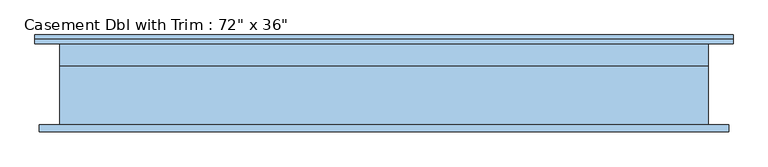
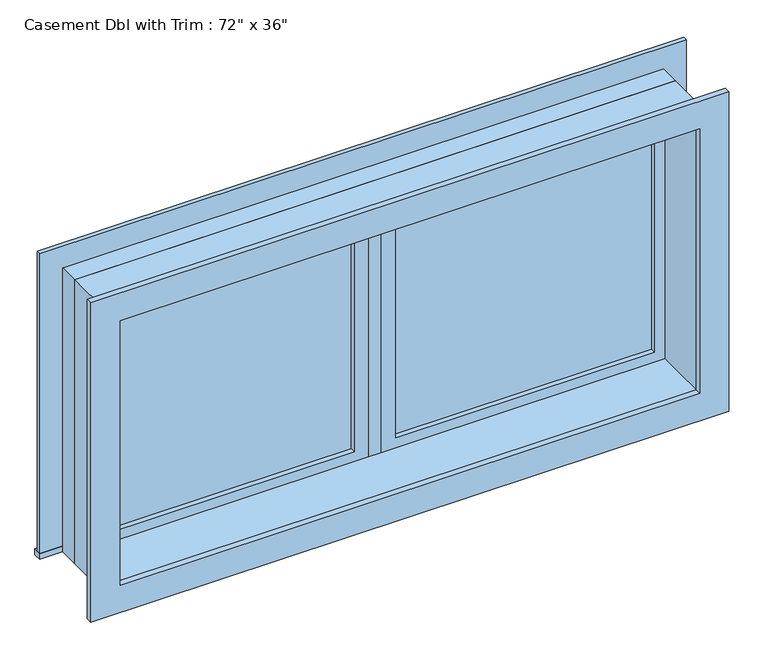
"""IFC4 building model written with IfcOpenShell, lengths in millimetres: window geometry."""

from ifc_helpers import new_model, si_unit, frame, origin, place, context, project, spatial, polyline, outline, extrude, source, transform, mapped, element, save


def window_6788402d(model_context):
    return source(origin(), model_context, "Body", "SweptSolid", [
        extrude(outline(polyline([(63.5, 98.425), (850.9, 98.425), (850.9, 85.725), (63.5, 85.725), (63.5, 98.425)])), frame((0.0, 0.0, 1282.7), z_axis=(0.0, 0.0, 1.0), x_axis=(1.0, 0.0, 0.0)), (0.0, 0.0, 1.0), 787.4),
        extrude(outline(polyline([(2114.55, 19.05), (1238.25, 19.05), (1238.25, 895.35), (2114.55, 895.35), (2114.55, 19.05)]), holes=[polyline([(2070.1, 63.5), (2070.1, 850.9), (1282.7, 850.9), (1282.7, 63.5), (2070.1, 63.5)])]), frame((0.0, 69.85, 0.0), z_axis=(0.0, 1.0, 0.0), x_axis=(0.0, 0.0, 1.0)), (0.0, 0.0, 1.0), 44.45),
        extrude(outline(polyline([(19.05, 69.85), (-19.05, 69.85), (-19.05, 133.35), (19.05, 133.35), (19.05, 69.85)])), frame((0.0, 0.0, 1238.25), z_axis=(0.0, 0.0, 1.0), x_axis=(1.0, 0.0, 0.0)), (0.0, 0.0, 1.0), 876.3),
        extrude(outline(polyline([(-984.25, 158.75), (984.25, 158.75), (984.25, 133.35), (-984.25, 133.35), (-984.25, 158.75)])), frame((0.0, 0.0, 1219.2), z_axis=(0.0, 0.0, 1.0), x_axis=(1.0, 0.0, 0.0)), (0.0, 0.0, 1.0), 19.05),
        extrude(outline(polyline([(2114.55, -895.35), (2114.55, 895.35), (1238.25, 895.35), (1238.25, 984.25), (2203.45, 984.25), (2203.45, -984.25), (1238.25, -984.25), (1238.25, -895.35), (2114.55, -895.35)])), frame((0.0, 133.35, 0.0), z_axis=(0.0, 1.0, 0.0), x_axis=(0.0, 0.0, 1.0)), (0.0, 0.0, 1.0), 12.7),
        extrude(outline(polyline([(2190.75, 971.55), (2190.75, -971.55), (1162.05, -971.55), (1162.05, 971.55), (2190.75, 971.55)]), holes=[polyline([(2101.85, 882.65), (1250.95, 882.65), (1250.95, -882.65), (2101.85, -882.65), (2101.85, 882.65)])]), frame((0.0, -114.3, 0.0), z_axis=(0.0, 1.0, 0.0), x_axis=(0.0, 0.0, 1.0)), (0.0, 0.0, 1.0), 19.05),
        extrude(outline(polyline([(-63.5, 85.725), (-850.9, 85.725), (-850.9, 98.425), (-63.5, 98.425), (-63.5, 85.725)])), frame((0.0, 0.0, 1282.7), z_axis=(0.0, 0.0, 1.0), x_axis=(1.0, 0.0, 0.0)), (0.0, 0.0, 1.0), 787.4),
        extrude(outline(polyline([(2114.55, -895.35), (1238.25, -895.35), (1238.25, -19.05), (2114.55, -19.05), (2114.55, -895.35)]), holes=[polyline([(2070.1, -850.9), (2070.1, -63.5), (1282.7, -63.5), (1282.7, -850.9), (2070.1, -850.9)])]), frame((0.0, 69.85, 0.0), z_axis=(0.0, 1.0, 0.0), x_axis=(0.0, 0.0, 1.0)), (0.0, 0.0, 1.0), 44.45),
        extrude(outline(polyline([(2133.6, -914.4), (1219.2, -914.4), (1219.2, 914.4), (2133.6, 914.4), (2133.6, -914.4)]), holes=[polyline([(2101.85, -882.65), (2101.85, 882.65), (1250.95, 882.65), (1250.95, -882.65), (2101.85, -882.65)])]), frame((0.0, -95.25, 0.0), z_axis=(0.0, 1.0, 0.0), x_axis=(0.0, 0.0, 1.0)), (0.0, 0.0, 1.0), 165.1),
        extrude(outline(polyline([(2133.6, 914.4), (2133.6, -914.4), (1219.2, -914.4), (1219.2, 914.4), (2133.6, 914.4)]), holes=[polyline([(2114.55, 895.35), (1238.25, 895.35), (1238.25, -895.35), (2114.55, -895.35), (2114.55, 895.35)])]), frame((0.0, 69.85, 0.0), z_axis=(0.0, 1.0, 0.0), x_axis=(0.0, 0.0, 1.0)), (0.0, 0.0, 1.0), 63.5),
    ])


if __name__ == "__main__":
    model = new_model("IFC4")
    model_context = context("Model", 3, world=origin())
    ifc_project = project(units=[si_unit("LENGTHUNIT", "METRE", prefix="MILLI")], contexts=[model_context])
    site = spatial("IfcSite", under=ifc_project)
    building = spatial("IfcBuilding", under=site)
    placement = place(None, origin())
    window_shape = window_6788402d(model_context)
    element("IfcWindow", 1, ObjectType="Casement Dbl with Trim : 72\" x 36\"", at=placement, inside=building, context=model_context, shape_type="MappedRepresentation", body=[
        mapped(window_shape, transform((0.0, 0.0, 0.0), x_axis=(1.0, 0.0, 0.0), y_axis=(0.0, 1.0, 0.0), z_axis=(0.0, 0.0, 1.0))),
    ])
    save(model, "model.ifc")

# Revit data of these elements
# Type "Casement Dbl with Trim : 72\" x 36\""
#   Type Mark = "11"
#   Construction Type Id = "GSP4R"
#   Assembly Code = "B2020100"
#   Analytic Construction = "1/8 in Pilkington single glazing"
#   Visual Light Transmittance = 0.9
#   Solar Heat Gain Coefficient = 0.78
#   Heat Transfer Coefficient (U) = 0.6496 BTU/(h·ft²·°F)
#   Height = 3' - 0"
#   Default Sill Height = 4' - 0"
#   Trim Projection - Ext. = 0' - 0 1/2"
#   Trim Projection - Int. = 0' - 0 3/4"
#   Trim Width - Exterior = 0' - 3 1/2"
#   Trim Width - Interior = 0' - 3 1/2"
#   Width = 6' - 0"
#   Window Inset = 0' - 0 3/4"
#   Define Thermal Properties by = 1
#   Glass Pane Material = Glass
#   Sash Material = Sash
#   Trim Exterior Material = Trim
#   Trim Interior Material = Trim
#   Wall Closure = (empty or 0)
# Element 1 (IfcWindow, "Casement Dbl with Trim : 72\" x 36\"")
#   Materials on its faces: "Sash", "Trim", "Glass"
# Materials
#   "Glass": class "Glass", colour RGB 0 128 192, transparency 0.75, Description = "Soda Lime Glass", Cost = 0
#   "Sash": class "Wood", colour RGB 224 178 126, transparency 0
#   "Trim": class "Wood", colour RGB 224 178 126, transparency 0
